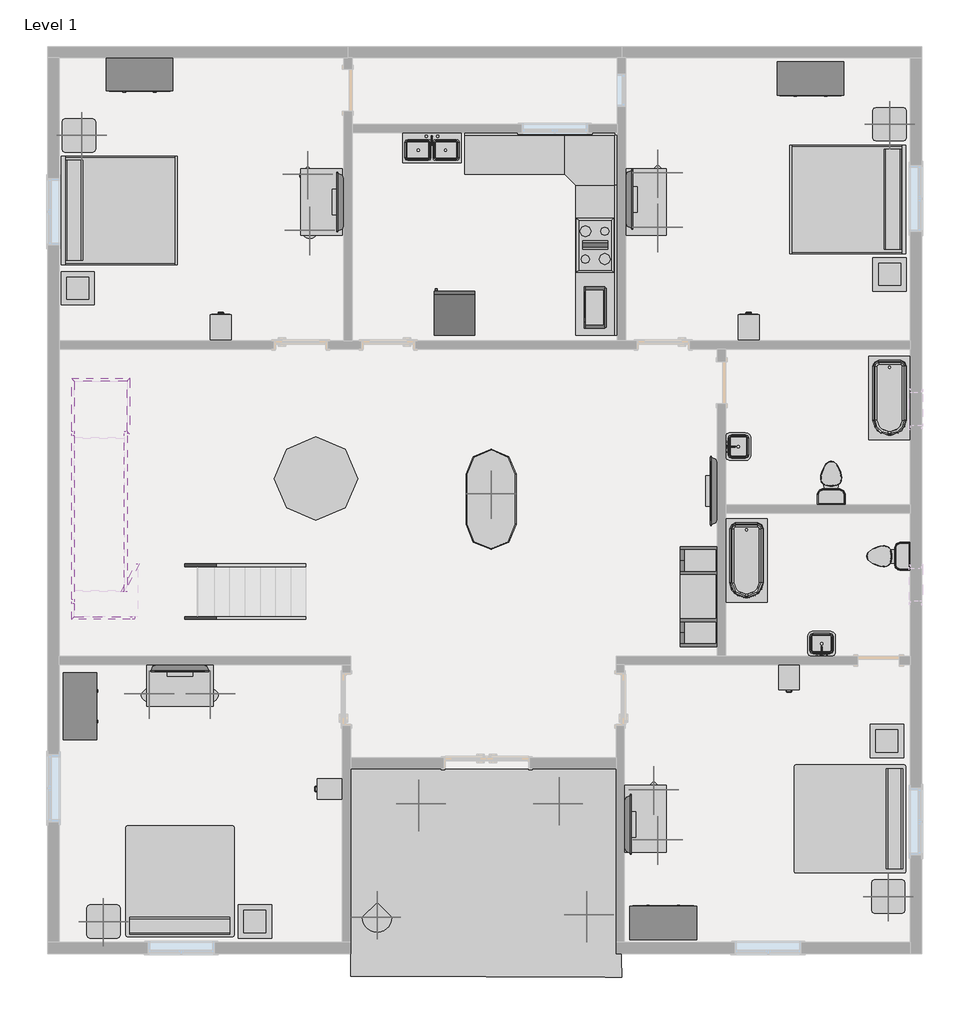
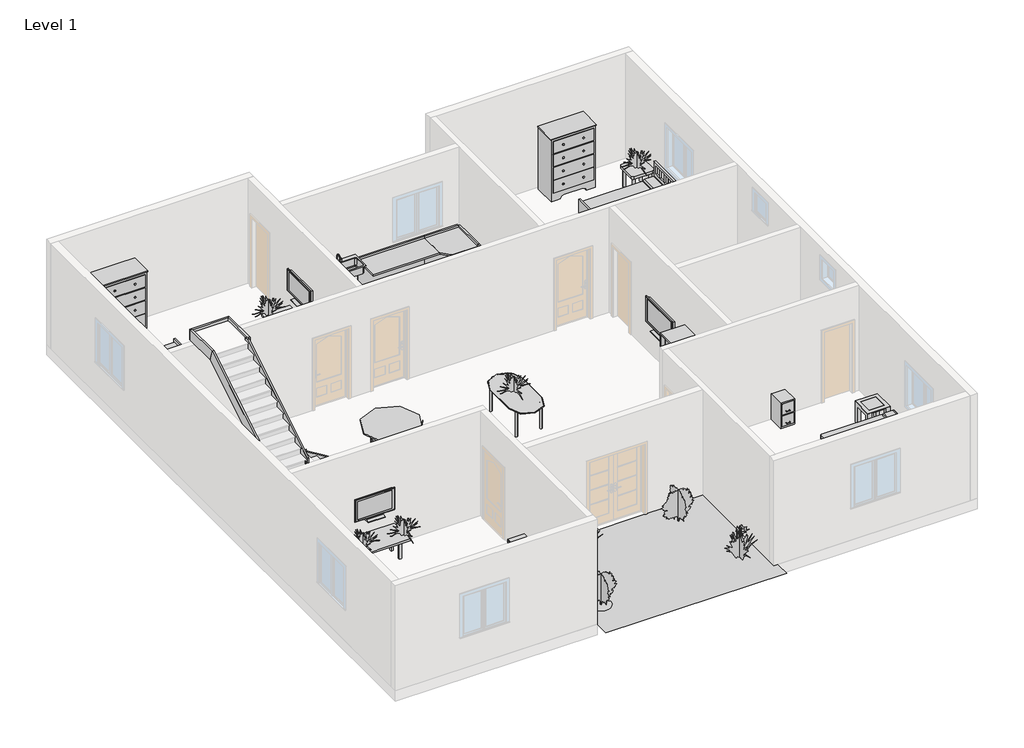
# One storey, part 2 of 2: 33 furniture elements, 17 geographic elements, 10 members, 9 flow terminals, 4 proxies.
"""IFC4 building model written with IfcOpenShell, lengths in millimetres."""

from ifc_helpers import new_model, si_unit, frame, origin, place, context, project, spatial, polyline, outline, extrude, faceted_brep, triangles, transform, mapped, element, save
from components import proxy_bb1e6e30, proxy_8a8d5ab2, proxy_a13a33b2, flow_terminal_accce45a, flow_terminal_a53be723, flow_terminal_62a433f7, toilet_domestic_3d_toilet_domestic_3d_f7549cf7, toilet_domestic_3d_toilet_domestic_3d_183bbd19, tub_rectangular_3d_tub_rectangular_3d_c1fa07c3, tub_rectangular_3d_tub_rectangular_3d_36e24cee, furniture_29cd36cd, furniture_1fc5af50, furniture_bb55ed6b, furniture_9fa109b2, furniture_cf0b6580, furniture_7a3aaa4f, furniture_fdf74506, furniture_b5c51a22, furniture_2c34a4f9, furniture_bbcc68ce, furniture_31d08a24, furniture_1bba2e14, furniture_452c495f, rpc_plant_tropical_55f6ff97, rpc_plant_tropical_agave_1_5_93a2a214, rpc_plant_tropical_jungle_flame_3_9c4808c2

model = new_model("IFC4")

# Units and contexts
model_context = context("Model", 3, world=origin())
ifc_project = project(units=[si_unit("LENGTHUNIT", "METRE", prefix="MILLI")], contexts=[model_context])

# Site, building, storey
site = spatial("IfcSite", under=ifc_project)
building = spatial("IfcBuilding", under=site)
storey = spatial("IfcBuildingStorey", under=building, Name="Level 1", Elevation=0.0)

# Proxies
placement = place(None, origin())
element("IfcBuildingElementProxy", 1, Name="Building Element Proxy", at=placement, inside=storey, context=model_context, shape_type="Tessellation", body=[
    triangles([(-9881.9828613, 1604.8620701, 0.0), (-5030.5830551, 1604.8620701, 0.0), (-5030.5830551, -1773.3379784, 0.0), (-9881.9828613, -1773.3379784, 0.0), (-4924.2430344, -2210.9018223, 0.0), (-9834.1706635, -2056.714286, 0.0), (-9885.9558746, -2188.959557, 0.0)], [[7, 4, 1], [4, 7, 6], [1, 4, 3], [6, 5, 3], [5, 6, 7], [2, 1, 3], [2, 3, 5], [3, 4, 6]], closed=False),
])
proxy_shape = proxy_bb1e6e30(model_context)
element("IfcBuildingElementProxy", 2, Name="Cook Top-4 Unit : 36\" x 20\"", ObjectType="Cook Top-4 Unit : 36\" x 20\"", at=placement, inside=storey, context=model_context, shape_type="MappedRepresentation", body=[
    mapped(proxy_shape, transform((-5411.58283, 11180.6620171, 0.0), x_axis=(0.0, 1.0000000000000002, 0.0), y_axis=(-1.0000000000000002, 0.0, 0.0), z_axis=(0.0, 0.0, 1.0))),
])
proxy_2_shape = proxy_8a8d5ab2(model_context)
element("IfcBuildingElementProxy", 3, Name="Microwave : 30\" x 16\" x 18\"", ObjectType="Microwave : 30\" x 16\" x 18\"", at=placement, inside=storey, context=model_context, shape_type="MappedRepresentation", body=[
    mapped(proxy_2_shape, transform((-5058.5023242, 10537.9548944, 0.0), x_axis=(0.0, -1.0000000000000002, 0.0), y_axis=(1.0000000000000002, 0.0, 0.0), z_axis=(0.0, 0.0, 1.0))),
])
proxy_3_shape = proxy_a13a33b2(model_context)
element("IfcBuildingElementProxy", 4, Name="Refrigerator : 30\" x 32\" RH", ObjectType="Refrigerator : 30\" x 32\" RH", at=placement, inside=storey, context=model_context, shape_type="MappedRepresentation", body=[
    mapped(proxy_3_shape, transform((-7984.92033, 9918.2109886, 0.0), x_axis=(-1.0000000000000004, 0.0, 0.0), y_axis=(0.0, -1.0000000000000004, 0.0), z_axis=(0.0, 0.0, 1.0))),
])

# Flow terminals
flow_terminal_shape = flow_terminal_accce45a(model_context)
element("IfcFlowTerminal", 5, ObjectType="Floor Drain - Round : 5\" Strainer - 2\" Drain", at=placement, inside=storey, context=model_context, shape_type="MappedRepresentation", body=[
    mapped(flow_terminal_shape, transform((-1322.18283, 9123.2620171, 0.0), x_axis=(1.0, 0.0, 0.0), y_axis=(0.0, 1.0, 0.0), z_axis=(0.0, 0.0, 1.0))),
])
element("IfcFlowTerminal", 6, ObjectType="Floor Drain - Round : 5\" Strainer - 2\" Drain", at=placement, inside=storey, context=model_context, shape_type="MappedRepresentation", body=[
    mapped(flow_terminal_shape, transform((49.41717, 4094.0620171, 0.0), x_axis=(1.0, 0.0, 0.0), y_axis=(0.0, 1.0, 0.0), z_axis=(0.0, 0.0, 1.0))),
])
flow_terminal_2_shape = flow_terminal_a53be723(model_context)
element("IfcFlowTerminal", 7, ObjectType="Sink Kitchen-Double : 42\" x 21\"", at=placement, inside=storey, context=model_context, shape_type="MappedRepresentation", body=[
    mapped(flow_terminal_2_shape, transform((-8411.7720705, 12956.316616, 0.0), x_axis=(1.0, 0.0, 0.0), y_axis=(0.0, 1.0, 0.0), z_axis=(0.0, 0.0, 1.0))),
])
flow_terminal_3_shape = flow_terminal_62a433f7(model_context)
element("IfcFlowTerminal", 8, ObjectType="Sink Vanity-Square : 20\" x 18\"", at=placement, inside=storey, context=model_context, shape_type="MappedRepresentation", body=[
    mapped(flow_terminal_3_shape, transform((-1255.6935894, 3842.4074182, 0.0), x_axis=(-1.0, 0.0, 0.0), y_axis=(0.0, -1.0, 0.0), z_axis=(0.0, 0.0, 1.0))),
])
element("IfcFlowTerminal", 9, ObjectType="Sink Vanity-Square : 20\" x 18\"", at=placement, inside=storey, context=model_context, shape_type="MappedRepresentation", body=[
    mapped(flow_terminal_3_shape, transform((-2843.8374289, 7481.9727765, 0.0), x_axis=(0.0, 1.0000000000000004, 0.0), y_axis=(-1.0000000000000004, 0.0, 0.0), z_axis=(0.0, 0.0, 1.0))),
])
toilet_domestic_3d_toilet_domestic_3d_shape = toilet_domestic_3d_toilet_domestic_3d_f7549cf7(model_context)
toilet_domestic_3d_toilet_domestic_3d_2_shape = toilet_domestic_3d_toilet_domestic_3d_183bbd19(model_context)
element("IfcFlowTerminal", 10, ObjectType="Toilet-Domestic-3D : Toilet-Domestic-3D", at=placement, inside=storey, context=model_context, shape_type="MappedRepresentation", body=[
    mapped(toilet_domestic_3d_toilet_domestic_3d_shape, transform((-1095.9091074, 6925.5580445, 0.0), x_axis=(-1.0000000000000004, 0.0, 0.0), y_axis=(0.0, -1.0000000000000004, 0.0), z_axis=(0.0, 0.0, 1.0))),
    mapped(toilet_domestic_3d_toilet_domestic_3d_2_shape, transform((-1095.9091074, 6925.5580445, 0.0), x_axis=(-1.0000000000000004, 0.0, 0.0), y_axis=(0.0, -1.0000000000000004, 0.0), z_axis=(0.0, 0.0, 1.0))),
])
element("IfcFlowTerminal", 11, ObjectType="Toilet-Domestic-3D : Toilet-Domestic-3D", at=placement, inside=storey, context=model_context, shape_type="MappedRepresentation", body=[
    mapped(toilet_domestic_3d_toilet_domestic_3d_shape, transform((-140.4788573, 5491.0620171, 0.0), x_axis=(0.0, -1.0, 0.0), y_axis=(1.0, 0.0, 0.0), z_axis=(0.0, 0.0, 1.0))),
    mapped(toilet_domestic_3d_toilet_domestic_3d_2_shape, transform((-140.4788573, 5491.0620171, 0.0), x_axis=(0.0, -1.0, 0.0), y_axis=(1.0, 0.0, 0.0), z_axis=(0.0, 0.0, 1.0))),
])
tub_rectangular_3d_tub_rectangular_3d_shape = tub_rectangular_3d_tub_rectangular_3d_c1fa07c3(model_context)
element("IfcFlowTerminal", 12, ObjectType="Tub-Rectangular-3D : Tub-Rectangular-3D", at=placement, inside=storey, context=model_context, shape_type="MappedRepresentation", body=[
    mapped(tub_rectangular_3d_tub_rectangular_3d_shape, transform((455.81717, 8038.0590484, 0.0), x_axis=(0.0, -1.0, 0.0), y_axis=(1.0, 0.0, 0.0), z_axis=(0.0, 0.0, 1.0))),
])
tub_rectangular_3d_tub_rectangular_3d_2_shape = tub_rectangular_3d_tub_rectangular_3d_36e24cee(model_context)
element("IfcFlowTerminal", 13, ObjectType="Tub-Rectangular-3D : Tub-Rectangular-3D", at=placement, inside=storey, context=model_context, shape_type="MappedRepresentation", body=[
    mapped(tub_rectangular_3d_tub_rectangular_3d_2_shape, transform((-3100.18283, 5066.2590484, 0.0), x_axis=(0.0, -1.0, 0.0), y_axis=(1.0, 0.0, 0.0), z_axis=(0.0, 0.0, 1.0))),
])

# Furniture
furniture_shape = furniture_29cd36cd(model_context)
element("IfcFurniture", 14, ObjectType="Bed-Shaker : King 78\" x 83\"", at=placement, inside=storey, context=model_context, shape_type="MappedRepresentation", body=[
    mapped(furniture_shape, transform((-15158.83283, 11834.7120171, 0.0), x_axis=(0.0, 1.0000000000000002, 0.0), y_axis=(-1.0000000000000002, 0.0, 0.0), z_axis=(0.0, 0.0, 1.0))),
])
element("IfcFurniture", 15, ObjectType="Bed-Shaker : King 78\" x 83\"", at=placement, inside=storey, context=model_context, shape_type="MappedRepresentation", body=[
    mapped(furniture_shape, transform((252.61717, 11999.8120171, 0.0), x_axis=(0.0, -1.0000000000000002, 0.0), y_axis=(1.0000000000000002, 0.0, 0.0), z_axis=(0.0, 0.0, 1.0))),
])
furniture_2_shape = furniture_1fc5af50(model_context)
element("IfcFurniture", 16, ObjectType="Bed-Standard : King 78\" x 80\"", at=placement, inside=storey, context=model_context, shape_type="MappedRepresentation", body=[
    mapped(furniture_2_shape, transform((-705.087748, 961.9505417, 0.0), x_axis=(0.0, -1.0000000000000009, 0.0), y_axis=(1.0000000000000009, 0.0, 0.0), z_axis=(0.0, 0.0, 1.0))),
])
element("IfcFurniture", 17, ObjectType="Bed-Standard : King 78\" x 80\"", at=placement, inside=storey, context=model_context, shape_type="MappedRepresentation", body=[
    mapped(furniture_2_shape, transform((-12734.6943054, -498.1330649, 0.0), x_axis=(-1.0000000000000004, 0.0, 0.0), y_axis=(0.0, -1.0000000000000004, 0.0), z_axis=(0.0, 0.0, 1.0))),
])
furniture_3_shape = furniture_bb55ed6b(model_context)
element("IfcFurniture", 18, ObjectType="Cabinet-File 2 Drawer : 15\" x 18\"", at=placement, inside=storey, context=model_context, shape_type="MappedRepresentation", body=[
    mapped(furniture_3_shape, transform((-12384.779277, 9539.927717, 0.0), x_axis=(-1.0000000000000002, 0.0, 0.0), y_axis=(0.0, -1.0000000000000002, 0.0), z_axis=(0.0, 0.0, 1.0))),
])
element("IfcFurniture", 19, ObjectType="Cabinet-File 2 Drawer : 15\" x 18\"", at=placement, inside=storey, context=model_context, shape_type="MappedRepresentation", body=[
    mapped(furniture_3_shape, transform((-2732.779277, 9539.927717, 0.0), x_axis=(-1.0000000000000002, 0.0, 0.0), y_axis=(0.0, -1.0000000000000002, 0.0), z_axis=(0.0, 0.0, 1.0))),
])
element("IfcFurniture", 20, ObjectType="Cabinet-File 2 Drawer : 15\" x 18\"", at=placement, inside=storey, context=model_context, shape_type="MappedRepresentation", body=[
    mapped(furniture_3_shape, transform((-1740.3863829, 3423.3963172, 0.0), x_axis=(1.0, 0.0, 0.0), y_axis=(0.0, 1.0, 0.0), z_axis=(0.0, 0.0, 1.0))),
])
element("IfcFurniture", 21, ObjectType="Cabinet-File 2 Drawer : 15\" x 18\"", at=placement, inside=storey, context=model_context, shape_type="MappedRepresentation", body=[
    mapped(furniture_3_shape, transform((-10120.8485299, 1108.6655701, 0.0), x_axis=(0.0, -1.0000000000000002, 0.0), y_axis=(1.0000000000000002, 0.0, 0.0), z_axis=(0.0, 0.0, 1.0))),
])
furniture_4_shape = furniture_9fa109b2(model_context)
element("IfcFurniture", 22, ObjectType="Dresser : 48\" x 72\" x 24\"", at=placement, inside=storey, context=model_context, shape_type="MappedRepresentation", body=[
    mapped(furniture_4_shape, transform((-13473.5895701, 14668.0249712, 0.0), x_axis=(1.0, 0.0, 0.0), y_axis=(0.0, 1.0, 0.0), z_axis=(0.0, 0.0, 1.0))),
])
element("IfcFurniture", 23, ObjectType="Dresser : 48\" x 72\" x 24\"", at=placement, inside=storey, context=model_context, shape_type="MappedRepresentation", body=[
    mapped(furniture_4_shape, transform((-1205.3895701, 14591.8249712, 0.0), x_axis=(1.0, 0.0, 0.0), y_axis=(0.0, 1.0, 0.0), z_axis=(0.0, 0.0, 1.0))),
])
element("IfcFurniture", 24, ObjectType="Dresser : 48\" x 72\" x 24\"", at=placement, inside=storey, context=model_context, shape_type="MappedRepresentation", body=[
    mapped(furniture_4_shape, transform((-4436.1760898, -1577.700937, 0.0), x_axis=(-1.0000000000000004, 0.0, 0.0), y_axis=(0.0, -1.0000000000000004, 0.0), z_axis=(0.0, 0.0, 1.0))),
])
element("IfcFurniture", 25, ObjectType="Dresser : 48\" x 72\" x 24\"", at=placement, inside=storey, context=model_context, shape_type="MappedRepresentation", body=[
    mapped(furniture_4_shape, transform((-15198.1457841, 3017.0552769, 0.0), x_axis=(0.0, 1.0, 0.0), y_axis=(-1.0, 0.0, 0.0), z_axis=(0.0, 0.0, 1.0))),
])
furniture_5_shape = furniture_cf0b6580(model_context)
element("IfcFurniture", 26, ObjectType="Entertainment Center : 72\" x 72\" x 24\"", at=placement, inside=storey, context=model_context, shape_type="MappedRepresentation", body=[
    mapped(furniture_5_shape, transform((-3074.78283, 4754.4620171, 0.0), x_axis=(0.0, -1.0000000000000004, 0.0), y_axis=(1.0000000000000004, 0.0, 0.0), z_axis=(0.0, 0.0, 1.0))),
])
furniture_6_shape = furniture_7a3aaa4f(model_context)
element("IfcFurniture", 27, ObjectType="TV - Flat Screen : 42\"", at=placement, inside=storey, context=model_context, shape_type="MappedRepresentation", body=[
    mapped(furniture_6_shape, transform((-10067.5214536, 11964.117503, 1041.4), x_axis=(0.0, -1.0000000000000004, 0.0), y_axis=(1.0000000000000004, 0.0, 0.0), z_axis=(0.0, 0.0, 1.0))),
])
element("IfcFurniture", 28, ObjectType="TV - Flat Screen : 42\"", at=placement, inside=storey, context=model_context, shape_type="MappedRepresentation", body=[
    mapped(furniture_6_shape, transform((-4794.2442063, 12022.8065313, 1041.4), x_axis=(0.0, 1.0000000000000002, 0.0), y_axis=(-1.0000000000000002, 0.0, 0.0), z_axis=(0.0, 0.0, 1.0))),
])
element("IfcFurniture", 29, ObjectType="TV - Flat Screen : 42\"", at=placement, inside=storey, context=model_context, shape_type="MappedRepresentation", body=[
    mapped(furniture_6_shape, transform((-4819.6442063, 592.8065313, 1041.4), x_axis=(0.0, 1.0000000000000002, 0.0), y_axis=(-1.0000000000000002, 0.0, 0.0), z_axis=(0.0, 0.0, 1.0))),
])
element("IfcFurniture", 30, ObjectType="TV - Flat Screen : 42\"", at=placement, inside=storey, context=model_context, shape_type="MappedRepresentation", body=[
    mapped(furniture_6_shape, transform((-13002.2383158, 3451.3233935, 1041.4), x_axis=(1.0, 0.0, 0.0), y_axis=(0.0, 1.0, 0.0), z_axis=(0.0, 0.0, 1.0))),
])
furniture_7_shape = furniture_fdf74506(model_context)
element("IfcFurniture", 31, ObjectType="TV - Flat Screen : 50\"", at=placement, inside=storey, context=model_context, shape_type="MappedRepresentation", body=[
    mapped(furniture_7_shape, transform((-3234.9214536, 6680.917503, 914.4), x_axis=(0.0, -1.0000000000000004, 0.0), y_axis=(1.0000000000000004, 0.0, 0.0), z_axis=(0.0, 0.0, 1.0))),
])
furniture_8_shape = furniture_b5c51a22(model_context)
element("IfcFurniture", 32, ObjectType="Table-Coffee : 24\" x 24\" x 24\"", at=placement, inside=storey, context=model_context, shape_type="MappedRepresentation", body=[
    mapped(furniture_8_shape, transform((-14891.3485967, 10298.0509393, 0.0), x_axis=(1.0, 0.0, 0.0), y_axis=(0.0, 1.0, 0.0), z_axis=(0.0, 0.0, 1.0))),
])
element("IfcFurniture", 33, ObjectType="Table-Coffee : 24\" x 24\" x 24\"", at=placement, inside=storey, context=model_context, shape_type="MappedRepresentation", body=[
    mapped(furniture_8_shape, transform((-45.0485967, 10552.0509393, 0.0), x_axis=(1.0, 0.0, 0.0), y_axis=(0.0, 1.0, 0.0), z_axis=(0.0, 0.0, 1.0))),
])
element("IfcFurniture", 34, ObjectType="Table-Coffee : 24\" x 24\" x 24\"", at=placement, inside=storey, context=model_context, shape_type="MappedRepresentation", body=[
    mapped(furniture_8_shape, transform((-95.8485967, 2017.6509393, 0.0), x_axis=(1.0, 0.0, 0.0), y_axis=(0.0, 1.0, 0.0), z_axis=(0.0, 0.0, 1.0))),
])
element("IfcFurniture", 35, ObjectType="Table-Coffee : 24\" x 24\" x 24\"", at=placement, inside=storey, context=model_context, shape_type="MappedRepresentation", body=[
    mapped(furniture_8_shape, transform((-11652.8485967, -1284.3490607, 0.0), x_axis=(1.0, 0.0, 0.0), y_axis=(0.0, 1.0, 0.0), z_axis=(0.0, 0.0, 1.0))),
])
furniture_9_shape = furniture_2c34a4f9(model_context)
element("IfcFurniture", 36, ObjectType="Table-Dining Oval : 36\" x 72\"", at=placement, inside=storey, context=model_context, shape_type="MappedRepresentation", body=[
    mapped(furniture_9_shape, transform((-7674.6811906, 6934.2816892, 0.0), x_axis=(0.0, 1.0, 0.0), y_axis=(-1.0, 0.0, 0.0), z_axis=(0.0, 0.0, 1.0))),
])
furniture_10_shape = furniture_bbcc68ce(model_context)
element("IfcFurniture", 37, ObjectType="Table-Dining Round w Chairs : 60\" Diameter", at=placement, inside=storey, context=model_context, shape_type="MappedRepresentation", body=[
    mapped(furniture_10_shape, transform((-10620.6647972, 7098.3407056, 0.0), x_axis=(1.0, 0.0, 0.0), y_axis=(0.0, 1.0, 0.0), z_axis=(0.0, 0.0, 1.0))),
])
furniture_11_shape = furniture_31d08a24(model_context)
element("IfcFurniture", 38, ObjectType="Table-End : 24\" x 24\"", at=placement, inside=storey, context=model_context, shape_type="MappedRepresentation", body=[
    mapped(furniture_11_shape, transform((-15162.5664603, 13034.8620171, 0.0), x_axis=(1.0, 0.0, 0.0), y_axis=(0.0, 1.0, 0.0), z_axis=(0.0, 0.0, 1.0))),
])
element("IfcFurniture", 39, ObjectType="Table-End : 24\" x 24\"", at=placement, inside=storey, context=model_context, shape_type="MappedRepresentation", body=[
    mapped(furniture_11_shape, transform((-335.3164603, 13238.0620171, 0.0), x_axis=(1.0, 0.0, 0.0), y_axis=(0.0, 1.0, 0.0), z_axis=(0.0, 0.0, 1.0))),
])
element("IfcFurniture", 40, ObjectType="Table-End : 24\" x 24\"", at=placement, inside=storey, context=model_context, shape_type="MappedRepresentation", body=[
    mapped(furniture_11_shape, transform((-360.7164603, -884.3379829, 0.0), x_axis=(1.0, 0.0, 0.0), y_axis=(0.0, 1.0, 0.0), z_axis=(0.0, 0.0, 1.0))),
])
element("IfcFurniture", 41, ObjectType="Table-End : 24\" x 24\"", at=placement, inside=storey, context=model_context, shape_type="MappedRepresentation", body=[
    mapped(furniture_11_shape, transform((-14711.7164603, -1341.5379829, 0.0), x_axis=(1.0, 0.0, 0.0), y_axis=(0.0, 1.0, 0.0), z_axis=(0.0, 0.0, 1.0))),
])
furniture_12_shape = furniture_1bba2e14(model_context)
element("IfcFurniture", 42, ObjectType="Table-Rectangular : 72\" x 30\"", at=placement, inside=storey, context=model_context, shape_type="MappedRepresentation", body=[
    mapped(furniture_12_shape, transform((-10415.38283, 11968.0620171, 0.0), x_axis=(0.0, 1.0000000000000002, 0.0), y_axis=(-1.0000000000000002, 0.0, 0.0), z_axis=(0.0, 0.0, 1.0))),
])
element("IfcFurniture", 43, ObjectType="Table-Rectangular : 72\" x 30\"", at=placement, inside=storey, context=model_context, shape_type="MappedRepresentation", body=[
    mapped(furniture_12_shape, transform((-4497.18283, 11968.0620171, 0.0), x_axis=(0.0, 1.0000000000000002, 0.0), y_axis=(-1.0000000000000002, 0.0, 0.0), z_axis=(0.0, 0.0, 1.0))),
])
element("IfcFurniture", 44, ObjectType="Table-Rectangular : 72\" x 30\"", at=placement, inside=storey, context=model_context, shape_type="MappedRepresentation", body=[
    mapped(furniture_12_shape, transform((-4497.18283, 690.4620171, 0.0), x_axis=(0.0, 1.0000000000000002, 0.0), y_axis=(-1.0000000000000002, 0.0, 0.0), z_axis=(0.0, 0.0, 1.0))),
])
element("IfcFurniture", 45, ObjectType="Table-Rectangular : 72\" x 30\"", at=placement, inside=storey, context=model_context, shape_type="MappedRepresentation", body=[
    mapped(furniture_12_shape, transform((-13006.18283, 3128.8620171, 0.0), x_axis=(1.0, 0.0, 0.0), y_axis=(0.0, 1.0, 0.0), z_axis=(0.0, 0.0, 1.0))),
])
furniture_13_shape = furniture_452c495f(model_context)
element("IfcFurniture", 46, ObjectType="Work Station Cubicle : 96\" x 96\"", at=placement, inside=storey, context=model_context, shape_type="MappedRepresentation", body=[
    mapped(furniture_13_shape, transform((-4510.1598224, 13106.3302649, 0.0), x_axis=(0.0, -1.0000000000000004, 0.0), y_axis=(1.0000000000000004, 0.0, 0.0), z_axis=(0.0, 0.0, 1.0))),
])

# Geographic elements
rpc_plant_tropical_shape = rpc_plant_tropical_55f6ff97(model_context)
element("IfcGeographicElement", 47, ObjectType="RPC Plant - Tropical", at=placement, inside=storey, context=model_context, shape_type="MappedRepresentation", body=[
    mapped(rpc_plant_tropical_shape, transform((-8637.38283, 969.8620171, 0.0), x_axis=(1.0, 0.0, 0.0), y_axis=(0.0, 1.0, 0.0), z_axis=(0.0, 0.0, 1.0))),
])
element("IfcGeographicElement", 48, ObjectType="RPC Plant - Tropical", at=placement, inside=storey, context=model_context, shape_type="MappedRepresentation", body=[
    mapped(rpc_plant_tropical_shape, transform((-5563.98283, -1062.1379829, 0.0), x_axis=(1.0, 0.0, 0.0), y_axis=(0.0, 1.0, 0.0), z_axis=(0.0, 0.0, 1.0))),
])
rpc_plant_tropical_agave_1_5_shape = rpc_plant_tropical_agave_1_5_93a2a214(model_context)
element("IfcGeographicElement", 49, ObjectType="RPC Plant - Tropical : Agave - 1.5'", at=placement, inside=storey, context=model_context, shape_type="MappedRepresentation", body=[
    mapped(rpc_plant_tropical_agave_1_5_shape, transform((-14803.23283, 13187.2620171, 609.6), x_axis=(1.0, 0.0, 0.0), y_axis=(0.0, 1.0, 0.0), z_axis=(0.0, 0.0, 1.0))),
])
element("IfcGeographicElement", 50, ObjectType="RPC Plant - Tropical : Agave - 1.5'", at=placement, inside=storey, context=model_context, shape_type="MappedRepresentation", body=[
    mapped(rpc_plant_tropical_agave_1_5_shape, transform((-10669.38283, 12476.0620171, 609.6), x_axis=(1.0, 0.0, 0.0), y_axis=(0.0, 1.0, 0.0), z_axis=(0.0, 0.0, 1.0))),
])
element("IfcGeographicElement", 51, ObjectType="RPC Plant - Tropical : Agave - 1.5'", at=placement, inside=storey, context=model_context, shape_type="MappedRepresentation", body=[
    mapped(rpc_plant_tropical_agave_1_5_shape, transform((-10631.28283, 11453.7120171, 609.6), x_axis=(1.0, 0.0, 0.0), y_axis=(0.0, 1.0, 0.0), z_axis=(0.0, 0.0, 1.0))),
])
element("IfcGeographicElement", 52, ObjectType="RPC Plant - Tropical : Agave - 1.5'", at=placement, inside=storey, context=model_context, shape_type="MappedRepresentation", body=[
    mapped(rpc_plant_tropical_agave_1_5_shape, transform((-26.78283, 13390.4620171, 609.6), x_axis=(1.0, 0.0, 0.0), y_axis=(0.0, 1.0, 0.0), z_axis=(0.0, 0.0, 1.0))),
])
element("IfcGeographicElement", 53, ObjectType="RPC Plant - Tropical : Agave - 1.5'", at=placement, inside=storey, context=model_context, shape_type="MappedRepresentation", body=[
    mapped(rpc_plant_tropical_agave_1_5_shape, transform((-4268.58283, 12501.4620171, 609.6), x_axis=(1.0, 0.0, 0.0), y_axis=(0.0, 1.0, 0.0), z_axis=(0.0, 0.0, 1.0))),
])
element("IfcGeographicElement", 54, ObjectType="RPC Plant - Tropical : Agave - 1.5'", at=placement, inside=storey, context=model_context, shape_type="MappedRepresentation", body=[
    mapped(rpc_plant_tropical_agave_1_5_shape, transform((-4268.58283, 11510.8620171, 609.6), x_axis=(1.0, 0.0, 0.0), y_axis=(0.0, 1.0, 0.0), z_axis=(0.0, 0.0, 1.0))),
])
element("IfcGeographicElement", 55, ObjectType="RPC Plant - Tropical : Agave - 1.5'", at=placement, inside=storey, context=model_context, shape_type="MappedRepresentation", body=[
    mapped(rpc_plant_tropical_agave_1_5_shape, transform((-52.18283, -731.9379829, 609.6), x_axis=(1.0, 0.0, 0.0), y_axis=(0.0, 1.0, 0.0), z_axis=(0.0, 0.0, 1.0))),
])
element("IfcGeographicElement", 56, ObjectType="RPC Plant - Tropical : Agave - 1.5'", at=placement, inside=storey, context=model_context, shape_type="MappedRepresentation", body=[
    mapped(rpc_plant_tropical_agave_1_5_shape, transform((-4344.78283, 1223.8620171, 609.6), x_axis=(1.0, 0.0, 0.0), y_axis=(0.0, 1.0, 0.0), z_axis=(0.0, 0.0, 1.0))),
])
element("IfcGeographicElement", 57, ObjectType="RPC Plant - Tropical : Agave - 1.5'", at=placement, inside=storey, context=model_context, shape_type="MappedRepresentation", body=[
    mapped(rpc_plant_tropical_agave_1_5_shape, transform((-4268.58283, 309.4620171, 609.6), x_axis=(1.0, 0.0, 0.0), y_axis=(0.0, 1.0, 0.0), z_axis=(0.0, 0.0, 1.0))),
])
element("IfcGeographicElement", 58, ObjectType="RPC Plant - Tropical : Agave - 1.5'", at=placement, inside=storey, context=model_context, shape_type="MappedRepresentation", body=[
    mapped(rpc_plant_tropical_agave_1_5_shape, transform((-14403.18283, -1189.1379829, 609.6), x_axis=(1.0, 0.0, 0.0), y_axis=(0.0, 1.0, 0.0), z_axis=(0.0, 0.0, 1.0))),
])
element("IfcGeographicElement", 59, ObjectType="RPC Plant - Tropical : Agave - 1.5'", at=placement, inside=storey, context=model_context, shape_type="MappedRepresentation", body=[
    mapped(rpc_plant_tropical_agave_1_5_shape, transform((-12447.38283, 2976.4620171, 609.6), x_axis=(1.0, 0.0, 0.0), y_axis=(0.0, 1.0, 0.0), z_axis=(0.0, 0.0, 1.0))),
])
element("IfcGeographicElement", 60, ObjectType="RPC Plant - Tropical : Agave - 1.5'", at=placement, inside=storey, context=model_context, shape_type="MappedRepresentation", body=[
    mapped(rpc_plant_tropical_agave_1_5_shape, transform((-13564.98283, 2976.4620171, 609.6), x_axis=(1.0, 0.0, 0.0), y_axis=(0.0, 1.0, 0.0), z_axis=(0.0, 0.0, 1.0))),
])
element("IfcGeographicElement", 61, ObjectType="RPC Plant - Tropical : Agave - 1.5'", at=placement, inside=storey, context=model_context, shape_type="MappedRepresentation", body=[
    mapped(rpc_plant_tropical_agave_1_5_shape, transform((-7316.58283, 6634.0620171, 736.6), x_axis=(1.0, 0.0, 0.0), y_axis=(0.0, 1.0, 0.0), z_axis=(0.0, 0.0, 1.0))),
])
rpc_plant_tropical_jungle_flame_3_shape = rpc_plant_tropical_jungle_flame_3_9c4808c2(model_context)
element("IfcGeographicElement", 62, ObjectType="RPC Plant - Tropical : Jungle Flame - 3'", at=placement, inside=storey, context=model_context, shape_type="MappedRepresentation", body=[
    mapped(rpc_plant_tropical_jungle_flame_3_shape, transform((-9399.38283, -1112.9379829, 0.0), x_axis=(1.0, 0.0, 0.0), y_axis=(0.0, 1.0, 0.0), z_axis=(0.0, 0.0, 1.0))),
])
element("IfcGeographicElement", 63, ObjectType="RPC Plant - Tropical : Jungle Flame - 3'", at=placement, inside=storey, context=model_context, shape_type="MappedRepresentation", body=[
    mapped(rpc_plant_tropical_jungle_flame_3_shape, transform((-6071.98283, 969.8620171, 0.0), x_axis=(1.0, 0.0, 0.0), y_axis=(0.0, 1.0, 0.0), z_axis=(0.0, 0.0, 1.0))),
])

# Members
element("IfcMember", 64, ObjectType="Stringer - 2\" Width", at=placement, inside=storey, context=model_context, shape_type="SweptSolid", body=[
    extrude(outline(polyline([(0.0, -10702.6822797), (212.114512, -10702.6822797), (2108.2, -13831.223335), (1803.4, -13916.3777915), (0.0, -10940.7677915), (0.0, -10702.6822797)])), frame((0.0, 4336.1500793, 0.0), z_axis=(0.0, 1.0, 0.0), x_axis=(0.0, 0.0, 1.0)), (0.0, 0.0, 1.0), 50.8),
])
element("IfcMember", 65, ObjectType="Stringer - 2\" Width", at=placement, inside=storey, context=model_context, shape_type="Brep", body=[
    faceted_brep([(-10702.6822797, 5352.1500793, 0.0), (-10702.6822797, 5301.3500793, 0.0), (-10940.7677915, 5301.3500793, 0.0), (-10940.7677915, 5352.1500793, 0.0), (-10702.6822797, 5352.1500793, 212.114512), (-10702.6822797, 5301.3500793, 212.114512), (-13748.7377742, 5352.1500793, 2058.208751), (-13776.0822797, 5301.3500793, 2074.7811786), (-13776.0822797, 5301.3500793, 1718.3724171), (-13748.7377742, 5352.1500793, 1701.7999895)], [[[0, 1, 2, 3]], [[4, 5, 1, 0]], [[5, 4, 6, 7]], [[1, 5, 7, 8, 2]], [[4, 0, 3, 9, 6]], [[2, 8, 9, 3]], [[6, 9, 8, 7]]]),
])
element("IfcMember", 66, ObjectType="Stringer - 2\" Width", at=placement, inside=storey, context=model_context, shape_type="SweptSolid", body=[
    extrude(outline(polyline([(4705.0455911, 1803.4), (4619.8911346, 2108.2), (7693.2911346, 3970.8666667), (7778.4455911, 3666.0666667), (4705.0455911, 1803.4)])), frame((-14987.38283, 0.0, 0.0), z_axis=(1.0, 0.0, 0.0), x_axis=(0.0, 1.0, 0.0)), (0.0, 0.0, 1.0), 50.8),
])
element("IfcMember", 67, ObjectType="Stringer - 2\" Width", at=placement, inside=storey, context=model_context, shape_type="SweptSolid", body=[
    extrude(outline(polyline([(4844.1500793, 1887.7057504), (4844.1500793, 2244.114512), (7693.2911346, 3970.8666667), (7777.0620171, 3970.8666667), (7777.0620171, 3665.228137), (4844.1500793, 1887.7057504)])), frame((-14022.18283, 0.0, 0.0), z_axis=(1.0, 0.0, 0.0), x_axis=(0.0, 1.0, 0.0)), (0.0, 0.0, 1.0), 50.8),
])
element("IfcMember", 68, ObjectType="Stringer - 2\" Width", at=placement, inside=storey, context=model_context, shape_type="Brep", body=[
    faceted_brep([(-14936.58283, 4619.8911346, 2108.2), (-14987.38283, 4619.8911346, 2108.2), (-14987.38283, 4336.1500793, 2108.2), (-14936.58283, 4386.9500793, 2108.2), (-14936.58283, 4705.0455911, 1803.4), (-14936.58283, 4386.9500793, 1803.4), (-14987.38283, 4705.0455911, 1803.4), (-14987.38283, 4336.1500793, 1803.4)], [[[0, 1, 2, 3]], [[4, 0, 3, 5]], [[6, 4, 5, 7]], [[1, 6, 7, 2]], [[1, 0, 4, 6]], [[2, 7, 5, 3]]]),
])
element("IfcMember", 69, ObjectType="Stringer - 2\" Width", at=placement, inside=storey, context=model_context, shape_type="Brep", body=[
    faceted_brep([(-14936.58283, 4386.9500793, 2108.2), (-14987.38283, 4336.1500793, 2108.2), (-13831.223335, 4336.1500793, 2108.2), (-13831.223335, 4386.9500793, 2108.2), (-14936.58283, 4386.9500793, 1803.4), (-13916.3777915, 4386.9500793, 1803.4), (-14987.38283, 4336.1500793, 1803.4), (-13916.3777915, 4336.1500793, 1803.4)], [[[0, 1, 2, 3]], [[4, 0, 3, 5]], [[6, 4, 5, 7]], [[1, 6, 7, 2]], [[1, 0, 4, 6]], [[2, 7, 5, 3]]]),
])
element("IfcMember", 70, ObjectType="Stringer - 2\" Width", at=placement, inside=storey, context=model_context, shape_type="SweptSolid", body=[
    extrude(outline(polyline([(-13806.4297319, 5352.1500793), (-13748.7377742, 5352.1500793), (-14022.18283, 4844.1500793), (-14079.8747877, 4844.1500793), (-13806.4297319, 5352.1500793)])), frame((0.0, 0.0, 1803.4), z_axis=(0.0, 0.0, 1.0), x_axis=(1.0, 0.0, 0.0)), (0.0, 0.0, 1.0), 304.8),
])
element("IfcMember", 71, ObjectType="Stringer - 2\" Width", at=placement, inside=storey, context=model_context, shape_type="SweptSolid", body=[
    extrude(outline(polyline([(-13920.58283, 7726.2620171), (-13971.38283, 7777.0620171), (-13971.38283, 8691.4620171), (-13920.58283, 8742.2620171), (-13920.58283, 7726.2620171)])), frame((0.0, 0.0, 3666.0666667), z_axis=(0.0, 0.0, 1.0), x_axis=(1.0, 0.0, 0.0)), (0.0, 0.0, 1.0), 304.8),
])
element("IfcMember", 72, ObjectType="Stringer - 2\" Width", at=placement, inside=storey, context=model_context, shape_type="SweptSolid", body=[
    extrude(outline(polyline([(-13920.58283, 8742.2620171), (-13971.38283, 8691.4620171), (-14936.58283, 8691.4620171), (-14987.38283, 8742.2620171), (-13920.58283, 8742.2620171)])), frame((0.0, 0.0, 3666.0666667), z_axis=(0.0, 0.0, 1.0), x_axis=(1.0, 0.0, 0.0)), (0.0, 0.0, 1.0), 304.8),
])
element("IfcMember", 73, ObjectType="Stringer - 2\" Width", at=placement, inside=storey, context=model_context, shape_type="Brep", body=[
    faceted_brep([(-14936.58283, 8691.4620171, 3970.8666667), (-14987.38283, 8742.2620171, 3970.8666667), (-14987.38283, 7693.2911346, 3970.8666667), (-14936.58283, 7693.2911346, 3970.8666667), (-14936.58283, 8691.4620171, 3666.0666667), (-14936.58283, 7778.4455911, 3666.0666667), (-14987.38283, 8742.2620171, 3666.0666667), (-14987.38283, 7778.4455911, 3666.0666667)], [[[0, 1, 2, 3]], [[4, 0, 3, 5]], [[6, 4, 5, 7]], [[1, 6, 7, 2]], [[1, 0, 4, 6]], [[2, 7, 5, 3]]]),
])

save(model, "model.ifc")

# Revit data of these elements
# Type "Cook Top-4 Unit : 36\" x 20\""
#   Assembly Code = "E1090400"
#   Depth = 2' - 0"
#   Width = 3' - 0"
#   Burner Material = Steel, Chrome Plated
#   Cooktop Material = Steel, Polished
#   Default Elevation = 0
# Type "Microwave : 30\" x 16\" x 18\""
#   Assembly Code = "E1090400"
#   Depth = 1' - 4"
#   Height = 1' - 6"
#   Width = 2' - 6"
#   Microwave Material = Laminate - Ivory, Glossy
#   Default Elevation = 0
# Type "Refrigerator : 30\" x 32\" RH"
#   Label = "REF."
#   Assembly Code = "E1090400"
#   Depth = 2' - 7 3/4"
#   Handle = 2' - 3"
#   Height = 5' - 10"
#   Rear Clearance = 0' - 2"
#   Top Door Height = 1' - 8"
#   Width = 2' - 5 3/8"
#   Material = Carpet (1)
#   Default Elevation = 0
# Type "Floor Drain - Round : 5\" Strainer - 2\" Drain"
#   WFU = 2
#   Strainer Height = 0' - 3 1/4"
#   Strainer Radius = 0' - 2 1/2"
#   Strainer Diameter = 0' - 5"
#   Radius 6 = 0' - 0 5/8"
#   Radius 5 = 0' - 1 1/4"
#   Radius 4 = 0' - 1 7/8"
#   Radius 2 = 0' - 3.04167"
#   Radius 1 = 0' - 2.02083"
#   Radius 3 = 0' - 2 1/32"
#   Pipe Radius = 1"
#   Pipe Diameter = 2"
#   Height 2 = 0' - 0.725"
#   Height 1 = 0' - 1 13/16"
#   Body Radius = 0' - 4 1/16"
#   Body Height = 0' - 3 5/8"
#   Body Diameter = 0' - 8 1/8"
#   Drain Material = none
#   HWFU = 0
#   Default Elevation = 0
#   CWFU = 0
# Type "Sink Kitchen-Double : 42\" x 21\""
#   Assembly Code = "D2010410"
#   Counter Height = 3' - 0"
#   Depth = 1' - 9"
#   Width = 3' - 6"
#   Faucet Material = Steel, Polished
#   Sink Material = Steel, Polished
#   Default Elevation = 0
# Type "Sink Vanity-Square : 20\" x 18\""
#   Assembly Code = "D2010400"
#   Counter Height = 2' - 7"
#   Depth = 1' - 6"
#   Width = 1' - 8"
#   Basin Material = Porcelain, Linen
#   Faucet Material = Steel, Polished
#   Default Elevation = 0
# Type "Toilet-Domestic-3D : Toilet-Domestic-3D"
#   Assembly Code = "D2010110"
#   Toilet - Bowl/Basin Material = Porcelain, Linen
#   Toilet - Seat Material = Laminate, Linen, Matte
#   Default Elevation = 0
# Type "Tub-Rectangular-3D : Tub-Rectangular-3D"
#   Assembly Code = "D2010500"
#   Depth = 2' - 6"
#   Height = 1' - 3"
#   Width = 5' - 0"
#   Tub Material = Porcelain, Ivory
#   Default Elevation = 0
# Type "Bed-Shaker : King 78\" x 83\""
#   Assembly Code = "E2020200"
#   Length = 6' - 11"
#   Width = 6' - 6"
#   Frame Material = Birch
#   Mattress Material = Softwood, Lumber
#   Default Elevation = 0
# Type "Bed-Standard : King 78\" x 80\""
#   Assembly Code = "E2020200"
#   Length = 6' - 8"
#   Width = 6' - 6"
#   Leg Material = Steel, Chrome Plated
#   Mattress Material = Linen, White
#   Default Elevation = 0
# Type "Cabinet-File 2 Drawer : 15\" x 18\""
#   Assembly Code = "E2020200"
#   Depth = 1' - 6"
#   Height = 2' - 5"
#   Width = 1' - 3"
#   Cabinet Material = Steel, Paint Finish, Ivory, Glossy
#   Handle Material = Steel, Chrome Plated
#   Default Elevation = 0
# Type "Dresser : 48\" x 72\" x 24\""
#   Assembly Code = "E2020200"
#   Depth = 2' - 0"
#   Height = 6' - 0"
#   Width = 4' - 0"
#   Dresser Material = Wood - Teak
#   Drawer Material = Wood - Teak
#   Knob Material = Cherry
#   Default Elevation = 0
# Type "Entertainment Center : 72\" x 72\" x 24\""
#   Assembly Code = "E2020200"
#   Center Width = 2' - 8"
#   Depth = 2' - 0"
#   Height = 6' - 0"
#   Width = 6' - 0"
#   Material = Wood - Teak
#   Default Elevation = 0
# Type "TV - Flat Screen : 42\""
#   SinAng = 0' - 0.0193"
#   L = 3' - 0.71517"
#   H = 1' - 8.65418"
#   Thickness = 0' - 4.33071"
#   Diagonal = 3' - 6.12598"
#   CosAng = 0' - 0.03431"
#   Stand [instance default] = yes
#   Default Elevation = 0
# Type "TV - Flat Screen : 50\""
#   SinAng = 0' - 0.0193"
#   L = 3' - 7.57782"
#   H = 2' - 0.51477"
#   Thickness = 0' - 4.33071"
#   Diagonal = 4' - 2"
#   CosAng = 0' - 0.03431"
#   Stand [instance default] = yes
#   Default Elevation = 0
# Type "Table-Coffee : 24\" x 24\" x 24\""
#   Assembly Code = "E2020200"
#   Height = 2' - 0"
#   Length = 2' - 0"
#   Width = 2' - 0"
#   Top Material = none
#   Frame Material = none
#   Default Elevation = 0
# Type "Table-Dining Oval : 36\" x 72\""
#   Assembly Code = "E2020200"
#   Length = 6' - 0"
#   Width = 3' - 0"
#   Base Material = Steel, Chrome Plated
#   Top Material = Glass - Clear, Grey
#   Default Elevation = 0
#   Description = (empty or 0)
# Type "Table-Dining Round w Chairs : 60\" Diameter"
#   Assembly Code = "E2020200"
#   Radius = 2' - 6"
#   Diameter = 5' - 0"
#   Height = 2' - 6"
#   Chairs = 6
#   Base Material = Pine
#   Top Material = Laminate, Linen, Matte
#   Default Elevation = 0
# Type "Table-End : 24\" x 24\""
#   Assembly Code = "E2020200"
#   Height = 2' - 0"
#   Length = 2' - 0"
#   Width = 2' - 0"
#   Base Material = Birch
#   Top Material = Laminate, Ivory, Matte
#   Default Elevation = 0
# Type "Table-Rectangular : 72\" x 30\""
#   Assembly Code = "E2020200"
#   Height = 2' - 0"
#   Length = 4' - 0"
#   Width = 2' - 6"
#   Base Material = Birch
#   Top Material = Birch
#   Default Elevation = 0
# Type "Work Station Cubicle : 96\" x 96\""
#   Assembly Code = "E2020"
#   Desktop Height = 2' - 6"
#   Desktop1 Width = 2' - 4"
#   Desktop2 Width = 2' - 4"
#   Panel Height = 2' - 8"
#   Panel1 Length = 6' - 0"
#   Panel2 Length = 9' - 0"
#   Cube Panel Material = Textile - Light Gray
#   Work Top Material = Laminate, Ivory, Matte
#   Default Elevation = 0
# Type "RPC Plant - Tropical"
#   built-in parameter 1005198 = "{2, 15},{39, RPC-16-FWM5-GM7X-C67P-4000-ST1L-LVER-AU},{1, 0},{1, 0},{2, 13},{1, 8},{5, Color},{1, 0},{1, 0},{3, 0.8},{3, 0.8},{3, 0.8},{1, 8},{7, BBoxMin},{1, 0},{1, 0},{1, 0},{1, 0},{1, 0},{1, 8},{7, BBoxMax},{1, 0},{1, 0},{1, 0},{1, 0},{1, 0},{2, 11},{9, RPCTypeId},{1, 0},{1, 0},{39, RPC-16-FWM5-GM7X-C67P-4000-ST1L-LVER-AU},{1, 6},{14, RPCPlantHeight},{1, 0},{1, 0},{1, 3},{2, 11},{7, keyword},{1, 0},{1, 0},{35, :RPCs:Shrubs [General]:Geometry:RPC},{2, 11},{8, category},{1, 0},{1, 0},{16, Shrubs [General]},{2, 11},{12, LocalizedUID},{1, 0},{1, 0},{10, Crane Lily},{2, 14},{6, Height},{1, 0},{1, 0},{1, 3},{1, 2},{16, Cast Reflections},{1, 0},{1, 0},{1, 0},{1, 2},{12, Cast Shadows},{1, 0},{1, 0},{1, 1},{1, 2},{9, Lock View},{1, 0},{1, 0},{1, 0},{1, 4},{5, ViewC},{1, 0},{1, 0},{1, 0},{21, assetlibrary_base.fbx},{1, 5},"
#   built-in parameter 1005195 = "RPC-16-FWM5-GM7X-C67P-4000-ST1L-LVER-AU"
#   Assembly Code = "G2050500"
#   Height = 3' - 0"
#   Default Elevation = 0
# Type "RPC Plant - Tropical : Agave - 1.5'"
#   built-in parameter 1005198 = "{2, 15},{39, RPC-16-G1GJ-63FX-7K5P-N000-ST1L-LVER-AU},{1, 0},{1, 0},{2, 13},{1, 8},{5, Color},{1, 0},{1, 0},{3, 0.8},{3, 0.8},{3, 0.8},{1, 8},{7, BBoxMin},{1, 0},{1, 0},{1, 0},{1, 0},{1, 0},{1, 8},{7, BBoxMax},{1, 0},{1, 0},{1, 0},{1, 0},{1, 0},{2, 11},{9, RPCTypeId},{1, 0},{1, 0},{39, RPC-16-G1GJ-63FX-7K5P-N000-ST1L-LVER-AU},{1, 6},{14, RPCPlantHeight},{1, 0},{1, 0},{3, 1.5},{2, 11},{7, keyword},{1, 0},{1, 0},{35, :RPCs:Plants [General]:Geometry:RPC},{2, 11},{8, category},{1, 0},{1, 0},{16, Plants [General]},{2, 11},{12, LocalizedUID},{1, 0},{1, 0},{5, Agave},{2, 14},{6, Height},{1, 0},{1, 0},{3, 1.5},{1, 2},{16, Cast Reflections},{1, 0},{1, 0},{1, 0},{1, 2},{12, Cast Shadows},{1, 0},{1, 0},{1, 1},{1, 2},{9, Lock View},{1, 0},{1, 0},{1, 0},{1, 4},{5, ViewC},{1, 0},{1, 0},{1, 0},{21, assetlibrary_base.fbx},{1, 5},"
#   built-in parameter 1005195 = "RPC-16-G1GJ-63FX-7K5P-N000-ST1L-LVER-AU"
#   Type Comments = "Agave"
#   Assembly Code = "G2050500"
#   Height = 1' - 6"
#   Default Elevation = 0
# Type "RPC Plant - Tropical : Jungle Flame - 3'"
#   built-in parameter 1005198 = "{2, 15},{39, RPC-16-FUVJ-JWG0-MWGK-8000-ST1L-LVER-AU},{1, 0},{1, 0},{2, 13},{1, 8},{5, Color},{1, 0},{1, 0},{3, 0.8},{3, 0.8},{3, 0.8},{1, 8},{7, BBoxMin},{1, 0},{1, 0},{1, 0},{1, 0},{1, 0},{1, 8},{7, BBoxMax},{1, 0},{1, 0},{1, 0},{1, 0},{1, 0},{2, 11},{9, RPCTypeId},{1, 0},{1, 0},{39, RPC-16-FUVJ-JWG0-MWGK-8000-ST1L-LVER-AU},{1, 6},{14, RPCPlantHeight},{1, 0},{1, 0},{1, 3},{2, 11},{7, keyword},{1, 0},{1, 0},{35, :RPCs:Shrubs [General]:Geometry:RPC},{2, 11},{8, category},{1, 0},{1, 0},{16, Shrubs [General]},{2, 11},{12, LocalizedUID},{1, 0},{1, 0},{12, Jungle Flame},{2, 14},{6, Height},{1, 0},{1, 0},{1, 3},{1, 2},{16, Cast Reflections},{1, 0},{1, 0},{1, 0},{1, 2},{12, Cast Shadows},{1, 0},{1, 0},{1, 1},{1, 2},{9, Lock View},{1, 0},{1, 0},{1, 0},{1, 4},{5, ViewC},{1, 0},{1, 0},{1, 0},{21, assetlibrary_base.fbx},{1, 5},"
#   built-in parameter 1005195 = "RPC-16-FUVJ-JWG0-MWGK-8000-ST1L-LVER-AU"
#   Type Comments = "Jungle Flame"
#   Assembly Code = "G2050500"
#   Height = 3' - 0"
#   Default Elevation = 0
# Element 1 (IfcBuildingElementProxy)
#   Material = Plant
#   Phase Created = New Construction
# Element 2 (IfcBuildingElementProxy, "Cook Top-4 Unit : 36\" x 20\"")
#   Phase Created = New Construction
#   Materials on its faces: "Steel, Chrome Plated", "Steel, Polished"
# Element 3 (IfcBuildingElementProxy, "Microwave : 30\" x 16\" x 18\"")
#   Phase Created = New Construction
#   Materials on its faces: "Laminate - Ivory, Glossy", "Glass"
# Element 4 (IfcBuildingElementProxy, "Refrigerator : 30\" x 32\" RH")
#   Phase Created = New Construction
#   Materials on its faces: "Carpet (1)", "Steel, Chrome Plated"
# Element 5 (IfcFlowTerminal, "Floor Drain - Round : 5\" Strainer - 2\" Drain")
#   Mark = "8"
#   Phase Created = New Construction
# Element 6 (IfcFlowTerminal, "Floor Drain - Round : 5\" Strainer - 2\" Drain")
#   Mark = "9"
#   Phase Created = New Construction
# Element 7 (IfcFlowTerminal, "Sink Kitchen-Double : 42\" x 21\"")
#   Mark = "1"
#   Phase Created = New Construction
#   Materials on its faces: "Steel, Polished"
# Element 8 (IfcFlowTerminal, "Sink Vanity-Square : 20\" x 18\"")
#   Mark = "6"
#   Phase Created = New Construction
#   Materials on its faces: "Porcelain, Linen", "Steel, Polished"
# Element 9 (IfcFlowTerminal, "Sink Vanity-Square : 20\" x 18\"")
#   Mark = "7"
#   Phase Created = New Construction
#   Materials on its faces: "Porcelain, Linen", "Steel, Polished"
# Element 10 (IfcFlowTerminal, "Toilet-Domestic-3D : Toilet-Domestic-3D")
#   Mark = "4"
#   Phase Created = New Construction
#   Materials on its faces: "Porcelain, Linen", "Laminate, Linen, Matte"
# Element 11 (IfcFlowTerminal, "Toilet-Domestic-3D : Toilet-Domestic-3D")
#   Mark = "5"
#   Phase Created = New Construction
#   Materials on its faces: "Porcelain, Linen", "Laminate, Linen, Matte"
# Element 12 (IfcFlowTerminal, "Tub-Rectangular-3D : Tub-Rectangular-3D")
#   Mark = "2"
#   Phase Created = New Construction
#   Materials on its faces: "Porcelain, Ivory"
# Element 13 (IfcFlowTerminal, "Tub-Rectangular-3D : Tub-Rectangular-3D")
#   Mark = "3"
#   Phase Created = New Construction
#   Materials on its faces: "Porcelain, Ivory"
# Elements 14, 15 (IfcFurniture, "Bed-Shaker : King 78\" x 83\"")
#   Phase Created = New Construction
#   Materials on its faces: "Birch", "Softwood, Lumber"
# Elements 16, 17 (IfcFurniture, "Bed-Standard : King 78\" x 80\"")
#   Phase Created = New Construction
#   Materials on its faces: "Linen, White", "Steel, Chrome Plated"
# Elements 18, 19, 20, 21 (IfcFurniture, "Cabinet-File 2 Drawer : 15\" x 18\"")
#   Phase Created = New Construction
#   Materials on its faces: "Steel, Chrome Plated", "Steel, Paint Finish, Ivory, Glossy"
# Elements 22, 23, 24, 25 (IfcFurniture, "Dresser : 48\" x 72\" x 24\"")
#   Phase Created = New Construction
#   Materials on its faces: "Laminate, Ivory, Matte", "Cherry", "Wood - Teak"
# Element 26 (IfcFurniture, "Entertainment Center : 72\" x 72\" x 24\"")
#   Phase Created = New Construction
#   Materials on its faces: "Wood - Teak", "Steel, Chrome Plated", "Glass - Clear, Grey"
# Elements 27, 28, 29, 30 (IfcFurniture, "TV - Flat Screen : 42\"")
#   Stand = yes
#   Phase Created = New Construction
#   Materials on its faces: "TV - Black", "TV - Glass", "TV - Screen"
# Element 31 (IfcFurniture, "TV - Flat Screen : 50\"")
#   Stand = yes
#   Phase Created = New Construction
#   Materials on its faces: "TV - Black", "TV - Glass", "TV - Screen"
# Elements 32, 33, 34, 35 (IfcFurniture, "Table-Coffee : 24\" x 24\" x 24\"")
#   Phase Created = New Construction
#   Materials on its faces: "Glass - Clear, Grey"
# Element 36 (IfcFurniture, "Table-Dining Oval : 36\" x 72\"")
#   Phase Created = New Construction
#   Materials on its faces: "Steel, Chrome Plated", "Glass - Clear, Grey"
# Element 37 (IfcFurniture, "Table-Dining Round w Chairs : 60\" Diameter")
#   Phase Created = New Construction
#   Materials on its faces: "Pine", "Laminate, Linen, Matte"
# Elements 38, 39, 40, 41 (IfcFurniture, "Table-End : 24\" x 24\"")
#   Phase Created = New Construction
#   Materials on its faces: "Laminate, Ivory, Matte", "Birch"
# Elements 42, 43, 44, 45 (IfcFurniture, "Table-Rectangular : 72\" x 30\"")
#   Phase Created = New Construction
#   Materials on its faces: "Birch"
# Element 46 (IfcFurniture, "Work Station Cubicle : 96\" x 96\"")
#   Phase Created = New Construction
#   Materials on its faces: "Textile - Light Gray", "Laminate, Ivory, Matte"
# Elements 47, 48 (IfcGeographicElement, "RPC Plant - Tropical")
#   Phase Created = New Construction
# Elements 49, 50, 51, 52, 53, 54, 55, 56, 57, 58, 59, 60, 61 (IfcGeographicElement, "RPC Plant - Tropical : Agave - 1.5'")
#   Phase Created = New Construction
# Elements 62, 63 (IfcGeographicElement, "RPC Plant - Tropical : Jungle Flame - 3'")
#   Phase Created = New Construction
# Elements 64, 65, 66, 67, 68, 69, 70, 71, 72, 73 (IfcMember, "Stringer - 2\" Width")
#   Phase Created = New Construction
# Materials
#   "Steel, Chrome Plated": class "Metal", colour RGB 17 17 17, transparency 0, Description = "Chromiuim plated steel", Cost = 0
#   "Steel, Polished": class "Metal", colour RGB 57 57 57, transparency 0, Description = "Polished steel", Cost = 0
#   "Laminate - Ivory, Glossy": colour RGB 247 247 239, transparency 0
#   "Carpet (1)": class "Carpet", colour RGB 124 80 67, transparency 0, Description = "Interior finish"
#   "Porcelain, Linen": class "Ceramic", colour RGB 249 239 230, transparency 0, Description = "Porcelain, linen", Cost = 0
#   "Laminate, Linen, Matte": class "Plastic", colour RGB 249 239 230, transparency 0, Description = "Plastic Laminate - Linen, Matte", Cost = 0
#   "Porcelain, Ivory": class "Ceramic", colour RGB 247 247 239, transparency 0, Description = "Porcelain, ivory", Cost = 0
#   "Birch": class "Wood", colour RGB 224 178 126, transparency 0, Description = "Betula Alleghaniensis", Cost = 0
#   "Softwood, Lumber": class "Wood", colour RGB 223 192 134, transparency 0, Description = "Pinus Echinata", Cost = 0
#   "Linen, White": class "Textile", colour RGB 247 247 239, transparency 0, Description = "Linen, white", Cost = 0
#   "Steel, Paint Finish, Ivory, Glossy": class "Metal", colour RGB 247 247 239, transparency 0, Description = "Steel, paint finish, ivory, glossy", Cost = 0
#   "Wood - Teak": class "Wood", colour RGB 145 112 90, transparency 0
#   "Cherry": class "Wood", colour RGB 226 177 128, transparency 0, Description = "Prunus Serotina", Cost = 0
#   "Glass - Clear, Grey": class "Glass", colour RGB 252 255 255, transparency 0.64
#   "Pine": class "Wood", colour RGB 223 192 134, transparency 0, Description = "Pinus Echinata", Cost = 0
#   "Laminate, Ivory, Matte": class "Plastic", colour RGB 247 247 239, transparency 0, Description = "Plastic Laminate - Ivory, Matte", Cost = 0
#   "Textile - Light Gray": class "Fabric", colour RGB 204 204 204, transparency 0
#   "Plant": class "Generic", colour RGB 0 0 0, transparency 0, Description = "physical material", Cost = 0
#   "Glass": class "Glass", colour RGB 0 128 192, transparency 0.75, Description = "Soda Lime Glass", Cost = 0
#   "TV - Black": colour RGB 49 49 49, transparency 0
#   "TV - Glass": colour RGB 157 157 157, transparency 0.9
#   "TV - Screen": colour RGB 0 0 0, transparency 0
